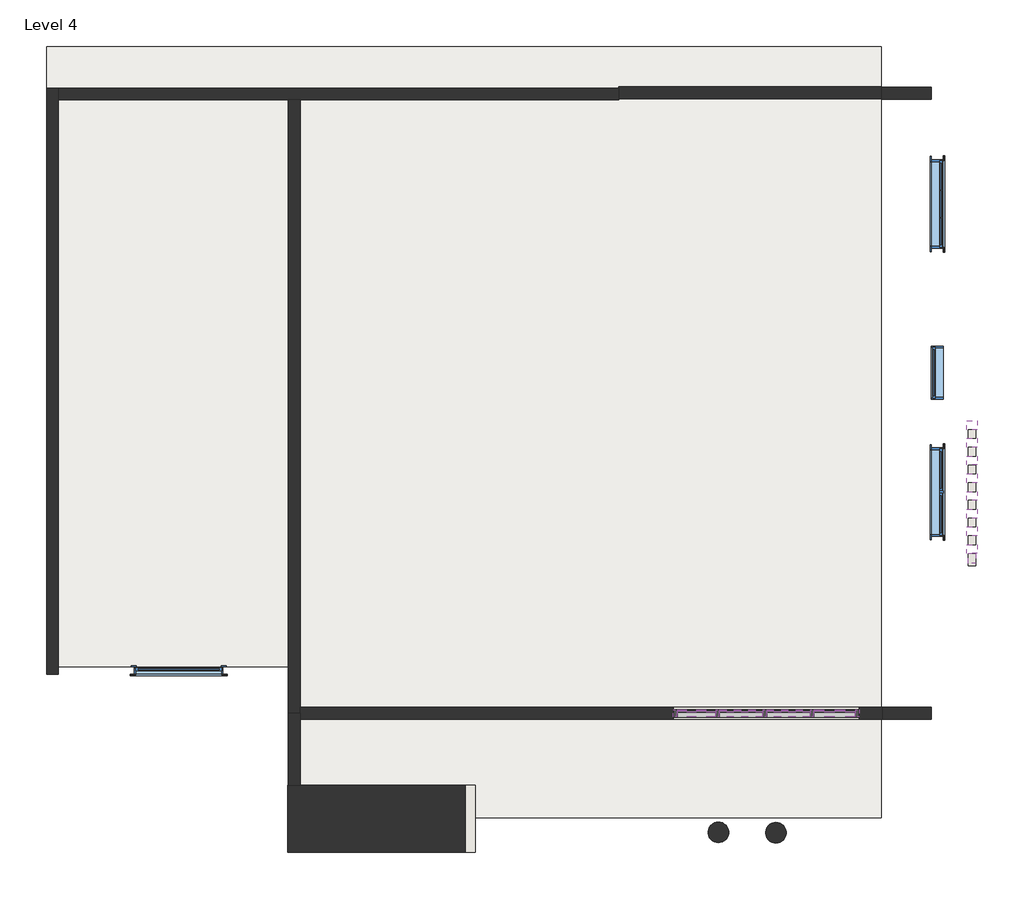
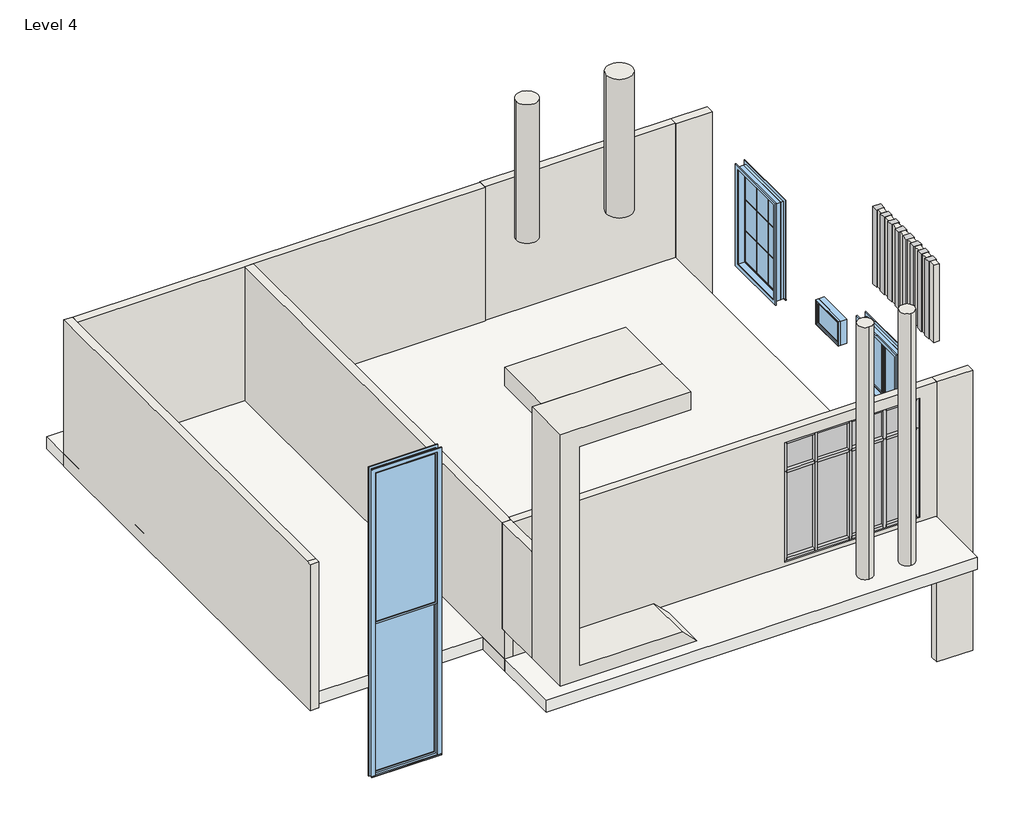
# One storey, incomplete: 22 members, 12 walls, 8 plates, 8 proxies, 4 windows, 1 roof.
"""IFC4 building model written with IfcOpenShell, lengths in millimetres."""

from ifc_helpers import new_model, si_unit, frame, origin, place, context, project, spatial, polyline, outline, extrude, faceted_brep, transform, mapped, element, save
from components import member_424e4c0f, member_61742b2b, member_5ade0aff, member_4d884067, member_c8ba4a72, member_20537117, member_aa870034, member_3a21dca5, member_2ee2964b, member_c33c434a, system_panel_glazed_10e47eeb, system_panel_glazed_d00a1739, system_panel_glazed_0ca22ccd, system_panel_glazed_ae16f783, system_panel_glazed_8c1b86c6, system_panel_glazed_afa25fb8, walls_4_walls_4_fad0a3e8, walls_5_walls_5_b947fde3, window_41dcc157, window_514a67b1, window_120b3672, window_57c3ee1c

model = new_model("IFC4")

# Units and contexts
model_context = context("Model", 3, world=origin())
ifc_project = project(units=[si_unit("LENGTHUNIT", "METRE", prefix="MILLI")], contexts=[model_context])

# Site, building, storey
site = spatial("IfcSite", under=ifc_project)
building = spatial("IfcBuilding", under=site)
storey = spatial("IfcBuildingStorey", under=building, Name="Level 4", Elevation=10972.8)

# Proxies
placement = place(None, origin())
element("IfcBuildingElementProxy", 1, Name="Reveal", ObjectType="Reveal", at=placement, inside=storey, context=model_context, shape_type="SweptSolid", body=[
    extrude(outline(polyline([(6653.2312442, 1993.3798743), (6470.3512442, 1993.3798743), (6470.3512442, 2145.7798743), (6653.2312442, 2145.7798743), (6653.2312442, 1993.3798743)])), frame((0.0, 0.0, 13469.4222175), z_axis=(0.0, 0.0, 1.0), x_axis=(1.0, 0.0, 0.0)), (0.0, 0.0, 1.0), 1931.5129026),
])
element("IfcBuildingElementProxy", 2, Name="Reveal", ObjectType="Reveal", at=placement, inside=storey, context=model_context, shape_type="SweptSolid", body=[
    extrude(outline(polyline([(6653.2312442, 2298.1798743), (6470.3512442, 2298.1798743), (6470.3512442, 2450.5798743), (6653.2312442, 2450.5798743), (6653.2312442, 2298.1798743)])), frame((0.0, 0.0, 13469.4222175), z_axis=(0.0, 0.0, 1.0), x_axis=(1.0, 0.0, 0.0)), (0.0, 0.0, 1.0), 1931.5129026),
])
element("IfcBuildingElementProxy", 3, Name="Reveal", ObjectType="Reveal", at=placement, inside=storey, context=model_context, shape_type="SweptSolid", body=[
    extrude(outline(polyline([(6653.2312442, 2602.9798743), (6470.3512442, 2602.9798743), (6470.3512442, 2755.3798743), (6653.2312442, 2755.3798743), (6653.2312442, 2602.9798743)])), frame((0.0, 0.0, 13469.4222175), z_axis=(0.0, 0.0, 1.0), x_axis=(1.0, 0.0, 0.0)), (0.0, 0.0, 1.0), 1931.5129026),
])
element("IfcBuildingElementProxy", 4, Name="Reveal", ObjectType="Reveal", at=placement, inside=storey, context=model_context, shape_type="SweptSolid", body=[
    extrude(outline(polyline([(6653.2312442, 2907.7798743), (6470.3512442, 2907.7798743), (6470.3512442, 3060.1798743), (6653.2312442, 3060.1798743), (6653.2312442, 2907.7798743)])), frame((0.0, 0.0, 13469.4222175), z_axis=(0.0, 0.0, 1.0), x_axis=(1.0, 0.0, 0.0)), (0.0, 0.0, 1.0), 1931.5129026),
])
element("IfcBuildingElementProxy", 5, Name="Reveal", ObjectType="Reveal", at=placement, inside=storey, context=model_context, shape_type="SweptSolid", body=[
    extrude(outline(polyline([(6653.2312442, 3212.5798743), (6470.3512442, 3212.5798743), (6470.3512442, 3364.9798743), (6653.2312442, 3364.9798743), (6653.2312442, 3212.5798743)])), frame((0.0, 0.0, 13469.4222175), z_axis=(0.0, 0.0, 1.0), x_axis=(1.0, 0.0, 0.0)), (0.0, 0.0, 1.0), 1931.5129026),
])
element("IfcBuildingElementProxy", 6, Name="Reveal", ObjectType="Reveal", at=placement, inside=storey, context=model_context, shape_type="SweptSolid", body=[
    extrude(outline(polyline([(6653.2312442, 3517.3798743), (6470.3512442, 3517.3798743), (6470.3512442, 3669.7798743), (6653.2312442, 3669.7798743), (6653.2312442, 3517.3798743)])), frame((0.0, 0.0, 13469.4222175), z_axis=(0.0, 0.0, 1.0), x_axis=(1.0, 0.0, 0.0)), (0.0, 0.0, 1.0), 1931.5129026),
])
element("IfcBuildingElementProxy", 7, Name="Reveal", ObjectType="Reveal", at=placement, inside=storey, context=model_context, shape_type="SweptSolid", body=[
    extrude(outline(polyline([(6653.2312442, 3822.1798743), (6470.3512442, 3822.1798743), (6470.3512442, 3974.5798743), (6653.2312442, 3974.5798743), (6653.2312442, 3822.1798743)])), frame((0.0, 0.0, 13469.4222175), z_axis=(0.0, 0.0, 1.0), x_axis=(1.0, 0.0, 0.0)), (0.0, 0.0, 1.0), 1931.5129026),
])
element("IfcBuildingElementProxy", 8, Name="Reveal", ObjectType="Reveal", at=placement, inside=storey, context=model_context, shape_type="SweptSolid", body=[
    extrude(outline(polyline([(6653.2312442, 4126.9798743), (6470.3512442, 4126.9798743), (6470.3512442, 4279.3798743), (6653.2312442, 4279.3798743), (6653.2312442, 4126.9798743)])), frame((0.0, 0.0, 13469.4222175), z_axis=(0.0, 0.0, 1.0), x_axis=(1.0, 0.0, 0.0)), (0.0, 0.0, 1.0), 1931.5129026),
])

# Members
member_shape = member_424e4c0f(model_context)
element("IfcMember", 9, ObjectType="Rectangular Mullion : 2.5\" x 5\" rectangular", at=placement, inside=storey, context=model_context, shape_type="MappedRepresentation", body=[
    mapped(member_shape, transform((3771.7551378, -759.3451257, 13606.9840877), x_axis=(0.0, 0.0, 1.0), y_axis=(0.0, -1.0, 0.0), z_axis=(1.0, 0.0, 0.0))),
])
element("IfcMember", 10, ObjectType="Rectangular Mullion : 2.5\" x 5\" rectangular", at=placement, inside=storey, context=model_context, shape_type="MappedRepresentation", body=[
    mapped(member_shape, transform((2958.9382617, -759.3451257, 13606.9840877), x_axis=(0.0, 0.0, 1.0), y_axis=(0.0, -1.0, 0.0), z_axis=(1.0, 0.0, 0.0))),
])
member_2_shape = member_61742b2b(model_context)
element("IfcMember", 11, ObjectType="Rectangular Mullion : 2.5\" x 5\" rectangular", at=placement, inside=storey, context=model_context, shape_type="MappedRepresentation", body=[
    mapped(member_2_shape, transform((2177.8713856, -759.3451257, 13606.9840877), x_axis=(1.0, 0.0, 0.0), y_axis=(0.0, -1.0, 0.0), z_axis=(0.0, 0.0, -1.0))),
])
element("IfcMember", 12, ObjectType="Rectangular Mullion : 2.5\" x 5\" rectangular", at=placement, inside=storey, context=model_context, shape_type="MappedRepresentation", body=[
    mapped(member_2_shape, transform((2990.6882617, -759.3451257, 13606.9840877), x_axis=(1.0, 0.0, 0.0), y_axis=(0.0, -1.0, 0.0), z_axis=(0.0, 0.0, -1.0))),
])
element("IfcMember", 13, ObjectType="Rectangular Mullion : 2.5\" x 5\" rectangular", at=placement, inside=storey, context=model_context, shape_type="MappedRepresentation", body=[
    mapped(member_2_shape, transform((3803.5051378, -759.3451257, 13606.9840877), x_axis=(1.0, 0.0, 0.0), y_axis=(0.0, -1.0, 0.0), z_axis=(0.0, 0.0, -1.0))),
])
member_3_shape = member_5ade0aff(model_context)
element("IfcMember", 14, ObjectType="Rectangular Mullion : 2.5\" x 5\" rectangular", at=placement, inside=storey, context=model_context, shape_type="MappedRepresentation", body=[
    mapped(member_3_shape, transform((3771.7551378, -759.3451257, 14368.9840877), x_axis=(0.0, 0.0, 1.0), y_axis=(0.0, -1.0, 0.0), z_axis=(1.0, 0.0, 0.0))),
])
element("IfcMember", 15, ObjectType="Rectangular Mullion : 2.5\" x 5\" rectangular", at=placement, inside=storey, context=model_context, shape_type="MappedRepresentation", body=[
    mapped(member_3_shape, transform((2958.9382617, -759.3451257, 14368.9840877), x_axis=(0.0, 0.0, 1.0), y_axis=(0.0, -1.0, 0.0), z_axis=(1.0, 0.0, 0.0))),
])
member_4_shape = member_4d884067(model_context)
element("IfcMember", 16, ObjectType="Rectangular Mullion : 2.5\" x 5\" rectangular", at=placement, inside=storey, context=model_context, shape_type="MappedRepresentation", body=[
    mapped(member_4_shape, transform((2177.8713856, -759.3451257, 11379.2), x_axis=(1.0, 0.0, 0.0), y_axis=(0.0, -1.0, 0.0), z_axis=(0.0, 0.0, -1.0))),
])
element("IfcMember", 17, ObjectType="Rectangular Mullion : 2.5\" x 5\" rectangular", at=placement, inside=storey, context=model_context, shape_type="MappedRepresentation", body=[
    mapped(member_4_shape, transform((2990.6882617, -759.3451257, 11379.2), x_axis=(1.0, 0.0, 0.0), y_axis=(0.0, -1.0, 0.0), z_axis=(0.0, 0.0, -1.0))),
])
element("IfcMember", 18, ObjectType="Rectangular Mullion : 2.5\" x 5\" rectangular", at=placement, inside=storey, context=model_context, shape_type="MappedRepresentation", body=[
    mapped(member_4_shape, transform((3803.5051378, -759.3451257, 11379.2), x_axis=(1.0, 0.0, 0.0), y_axis=(0.0, -1.0, 0.0), z_axis=(0.0, 0.0, -1.0))),
])
element("IfcMember", 19, ObjectType="Rectangular Mullion : 2.5\" x 5\" rectangular", at=placement, inside=storey, context=model_context, shape_type="MappedRepresentation", body=[
    mapped(member_3_shape, transform((3022.4382617, -759.3451257, 11379.2), x_axis=(0.0, 0.0, -1.0), y_axis=(0.0, -1.0, 0.0), z_axis=(-1.0, 0.0, 0.0))),
])
element("IfcMember", 20, ObjectType="Rectangular Mullion : 2.5\" x 5\" rectangular", at=placement, inside=storey, context=model_context, shape_type="MappedRepresentation", body=[
    mapped(member_3_shape, transform((2209.6213856, -759.3451257, 11379.2), x_axis=(0.0, 0.0, -1.0), y_axis=(0.0, -1.0, 0.0), z_axis=(-1.0, 0.0, 0.0))),
])
member_5_shape = member_c8ba4a72(model_context)
element("IfcMember", 21, ObjectType="Rectangular Mullion : 2.5\" x 5\" rectangular", at=placement, inside=storey, context=model_context, shape_type="MappedRepresentation", body=[
    mapped(member_5_shape, transform((4552.8220139, -759.3451257, 13606.9840877), x_axis=(0.0, 0.0, 1.0), y_axis=(0.0, -1.0, 0.0), z_axis=(1.0, 0.0, 0.0))),
])
member_6_shape = member_20537117(model_context)
element("IfcMember", 22, ObjectType="Rectangular Mullion : 2.5\" x 5\" rectangular", at=placement, inside=storey, context=model_context, shape_type="MappedRepresentation", body=[
    mapped(member_6_shape, transform((4552.8220139, -759.3451257, 14368.9840877), x_axis=(0.0, 0.0, 1.0), y_axis=(0.0, -1.0, 0.0), z_axis=(1.0, 0.0, 0.0))),
])
element("IfcMember", 23, ObjectType="Rectangular Mullion : 2.5\" x 5\" rectangular", at=placement, inside=storey, context=model_context, shape_type="MappedRepresentation", body=[
    mapped(member_6_shape, transform((3835.2551378, -759.3451257, 11379.2), x_axis=(0.0, 0.0, -1.0), y_axis=(0.0, -1.0, 0.0), z_axis=(-1.0, 0.0, 0.0))),
])
member_7_shape = member_aa870034(model_context)
element("IfcMember", 24, ObjectType="Rectangular Mullion : 2.5\" x 5\" rectangular", at=placement, inside=storey, context=model_context, shape_type="MappedRepresentation", body=[
    mapped(member_7_shape, transform((4616.3220139, -759.3451257, 13606.9840877), x_axis=(1.0, 0.0, 0.0), y_axis=(0.0, -1.0, 0.0), z_axis=(0.0, 0.0, -1.0))),
])
member_8_shape = member_3a21dca5(model_context)
element("IfcMember", 25, ObjectType="Rectangular Mullion : 2.5\" x 5\" rectangular", at=placement, inside=storey, context=model_context, shape_type="MappedRepresentation", body=[
    mapped(member_8_shape, transform((4616.3220139, -759.3451257, 11379.2), x_axis=(1.0, 0.0, 0.0), y_axis=(0.0, -1.0, 0.0), z_axis=(0.0, 0.0, -1.0))),
])
member_9_shape = member_2ee2964b(model_context)
element("IfcMember", 26, ObjectType="Rectangular Mullion : 2.5\" x 5\" rectangular", at=placement, inside=storey, context=model_context, shape_type="MappedRepresentation", body=[
    mapped(member_9_shape, transform((2146.1213856, -759.3451257, 13606.9840877), x_axis=(0.0, 0.0, 1.0), y_axis=(0.0, -1.0, 0.0), z_axis=(1.0, 0.0, 0.0))),
])
member_10_shape = member_c33c434a(model_context)
element("IfcMember", 27, ObjectType="Rectangular Mullion : 2.5\" x 5\" rectangular", at=placement, inside=storey, context=model_context, shape_type="MappedRepresentation", body=[
    mapped(member_10_shape, transform((2146.1213856, -759.3451257, 14368.9840877), x_axis=(0.0, 0.0, 1.0), y_axis=(0.0, -1.0, 0.0), z_axis=(1.0, 0.0, 0.0))),
])
element("IfcMember", 28, ObjectType="Rectangular Mullion : 2.5\" x 5\" rectangular", at=placement, inside=storey, context=model_context, shape_type="MappedRepresentation", body=[
    mapped(member_10_shape, transform((1479.3713856, -759.3451257, 11379.2), x_axis=(0.0, 0.0, -1.0), y_axis=(0.0, -1.0, 0.0), z_axis=(-1.0, 0.0, 0.0))),
])
element("IfcMember", 29, ObjectType="Rectangular Mullion : 2.5\" x 5\" rectangular", at=placement, inside=storey, context=model_context, shape_type="MappedRepresentation", body=[
    mapped(member_8_shape, transform((1415.8713856, -759.3451257, 13606.9840877), x_axis=(-1.0, 0.0, 0.0), y_axis=(0.0, -1.0, 0.0), z_axis=(0.0, 0.0, 1.0))),
])
element("IfcMember", 30, ObjectType="Rectangular Mullion : 2.5\" x 5\" rectangular", at=placement, inside=storey, context=model_context, shape_type="MappedRepresentation", body=[
    mapped(member_7_shape, transform((1415.8713856, -759.3451257, 14368.9840877), x_axis=(-1.0, 0.0, 0.0), y_axis=(0.0, -1.0, 0.0), z_axis=(0.0, 0.0, 1.0))),
])

# Plates
system_panel_glazed_shape = system_panel_glazed_10e47eeb(model_context)
element("IfcPlate", 31, ObjectType="System Panel : Glazed", at=placement, inside=storey, context=model_context, shape_type="MappedRepresentation", body=[
    mapped(system_panel_glazed_shape, transform((2584.2798237, -759.3451257, 13638.7340877), x_axis=(1.0, 0.0, 0.0), y_axis=(0.0, 1.0, 0.0), z_axis=(0.0, 0.0, 1.0))),
])
element("IfcPlate", 32, ObjectType="System Panel : Glazed", at=placement, inside=storey, context=model_context, shape_type="MappedRepresentation", body=[
    mapped(system_panel_glazed_shape, transform((3397.0966998, -759.3451257, 13638.7340877), x_axis=(1.0, 0.0, 0.0), y_axis=(0.0, 1.0, 0.0), z_axis=(0.0, 0.0, 1.0))),
])
system_panel_glazed_2_shape = system_panel_glazed_d00a1739(model_context)
element("IfcPlate", 33, ObjectType="System Panel : Glazed", at=placement, inside=storey, context=model_context, shape_type="MappedRepresentation", body=[
    mapped(system_panel_glazed_2_shape, transform((2584.2798237, -759.3451257, 11442.7), x_axis=(1.0, 0.0, 0.0), y_axis=(0.0, 1.0, 0.0), z_axis=(0.0, 0.0, 1.0))),
])
element("IfcPlate", 34, ObjectType="System Panel : Glazed", at=placement, inside=storey, context=model_context, shape_type="MappedRepresentation", body=[
    mapped(system_panel_glazed_2_shape, transform((3397.0966998, -759.3451257, 11442.7), x_axis=(1.0, 0.0, 0.0), y_axis=(0.0, 1.0, 0.0), z_axis=(0.0, 0.0, 1.0))),
])
system_panel_glazed_3_shape = system_panel_glazed_0ca22ccd(model_context)
element("IfcPlate", 35, ObjectType="System Panel : Glazed", at=placement, inside=storey, context=model_context, shape_type="MappedRepresentation", body=[
    mapped(system_panel_glazed_3_shape, transform((4194.0385758, -759.3451257, 11442.7), x_axis=(1.0, 0.0, 0.0), y_axis=(0.0, 1.0, 0.0), z_axis=(0.0, 0.0, 1.0))),
])
system_panel_glazed_4_shape = system_panel_glazed_ae16f783(model_context)
element("IfcPlate", 36, ObjectType="System Panel : Glazed", at=placement, inside=storey, context=model_context, shape_type="MappedRepresentation", body=[
    mapped(system_panel_glazed_4_shape, transform((4194.0385758, -759.3451257, 13638.7340877), x_axis=(1.0, 0.0, 0.0), y_axis=(0.0, 1.0, 0.0), z_axis=(0.0, 0.0, 1.0))),
])
system_panel_glazed_5_shape = system_panel_glazed_8c1b86c6(model_context)
element("IfcPlate", 37, ObjectType="System Panel : Glazed", at=placement, inside=storey, context=model_context, shape_type="MappedRepresentation", body=[
    mapped(system_panel_glazed_5_shape, transform((1812.7463856, -759.3451257, 11442.7), x_axis=(1.0, 0.0, 0.0), y_axis=(0.0, 1.0, 0.0), z_axis=(0.0, 0.0, 1.0))),
])
system_panel_glazed_6_shape = system_panel_glazed_afa25fb8(model_context)
element("IfcPlate", 38, ObjectType="System Panel : Glazed", at=placement, inside=storey, context=model_context, shape_type="MappedRepresentation", body=[
    mapped(system_panel_glazed_6_shape, transform((1812.7463856, -759.3451257, 13638.7340877), x_axis=(1.0, 0.0, 0.0), y_axis=(0.0, 1.0, 0.0), z_axis=(0.0, 0.0, 1.0))),
])

# Roof
element("IfcRoof", 39, ObjectType="Generic - 12\"", at=placement, inside=storey, context=model_context, shape_type="SweptSolid", body=[
    extrude(outline(polyline([(-9379.3749149, 10724.4481987), (4997.0250851, 10724.4481987), (4997.0250851, -2559.7518013), (-5213.7749149, -2559.7518013), (-5213.7749149, 40.7548743), (-9379.3749149, 40.7548743), (-9379.3749149, 10724.4481987)])), frame((0.0, 0.0, 10972.8), z_axis=(0.0, 0.0, 1.0), x_axis=(1.0, 0.0, 0.0)), (0.0, 0.0, 1.0), 304.8),
])

# Walls
element("IfcWall", 40, ObjectType="Generic - 5\"", at=placement, inside=storey, context=model_context, shape_type="SweptSolid", body=[
    extrude(outline(polyline([(6622.7512442, 1824.7794951), (6495.7512442, 1824.7794951), (6495.7512442, 1993.3798743), (6622.7512442, 1993.3798743), (6622.7512442, 1824.7794951)])), frame((0.0, 0.0, 13469.4222175), z_axis=(0.0, 0.0, 1.0), x_axis=(1.0, 0.0, 0.0)), (0.0, 0.0, 1.0), 1931.5129026),
    extrude(outline(polyline([(6622.7512442, 2145.7798743), (6495.7512442, 2145.7798743), (6495.7512442, 2298.1798743), (6622.7512442, 2298.1798743), (6622.7512442, 2145.7798743)])), frame((0.0, 0.0, 13469.4222175), z_axis=(0.0, 0.0, 1.0), x_axis=(1.0, 0.0, 0.0)), (0.0, 0.0, 1.0), 1931.5129026),
    extrude(outline(polyline([(6622.7512442, 2450.5798743), (6495.7512442, 2450.5798743), (6495.7512442, 2602.9798743), (6622.7512442, 2602.9798743), (6622.7512442, 2450.5798743)])), frame((0.0, 0.0, 13469.4222175), z_axis=(0.0, 0.0, 1.0), x_axis=(1.0, 0.0, 0.0)), (0.0, 0.0, 1.0), 1931.5129026),
    extrude(outline(polyline([(6622.7512442, 2755.3798743), (6495.7512442, 2755.3798743), (6495.7512442, 2907.7798743), (6622.7512442, 2907.7798743), (6622.7512442, 2755.3798743)])), frame((0.0, 0.0, 13469.4222175), z_axis=(0.0, 0.0, 1.0), x_axis=(1.0, 0.0, 0.0)), (0.0, 0.0, 1.0), 1931.5129026),
    extrude(outline(polyline([(6622.7512442, 3060.1798743), (6495.7512442, 3060.1798743), (6495.7512442, 3212.5798743), (6622.7512442, 3212.5798743), (6622.7512442, 3060.1798743)])), frame((0.0, 0.0, 13469.4222175), z_axis=(0.0, 0.0, 1.0), x_axis=(1.0, 0.0, 0.0)), (0.0, 0.0, 1.0), 1931.5129026),
    extrude(outline(polyline([(6622.7512442, 3364.9798743), (6495.7512442, 3364.9798743), (6495.7512442, 3517.3798743), (6622.7512442, 3517.3798743), (6622.7512442, 3364.9798743)])), frame((0.0, 0.0, 13469.4222175), z_axis=(0.0, 0.0, 1.0), x_axis=(1.0, 0.0, 0.0)), (0.0, 0.0, 1.0), 1931.5129026),
    extrude(outline(polyline([(6622.7512442, 3669.7798743), (6495.7512442, 3669.7798743), (6495.7512442, 3822.1798743), (6622.7512442, 3822.1798743), (6622.7512442, 3669.7798743)])), frame((0.0, 0.0, 13469.4222175), z_axis=(0.0, 0.0, 1.0), x_axis=(1.0, 0.0, 0.0)), (0.0, 0.0, 1.0), 1931.5129026),
    extrude(outline(polyline([(6622.7512442, 3974.5798743), (6495.7512442, 3974.5798743), (6495.7512442, 4126.9798743), (6622.7512442, 4126.9798743), (6622.7512442, 3974.5798743)])), frame((0.0, 0.0, 13469.4222175), z_axis=(0.0, 0.0, 1.0), x_axis=(1.0, 0.0, 0.0)), (0.0, 0.0, 1.0), 1931.5129026),
])
element("IfcWall", 41, ObjectType="Generic - 5\"", at=placement, inside=storey, context=model_context, shape_type="SweptSolid", body=[
    extrude(outline(polyline([(6622.7512442, 1784.3255336), (6495.7512442, 1784.3255336), (6495.7512442, 1993.3798743), (6622.7512442, 1993.3798743), (6622.7512442, 1784.3255336)])), frame((0.0, 0.0, 7620.0), z_axis=(0.0, 0.0, 1.0), x_axis=(1.0, 0.0, 0.0)), (0.0, 0.0, 1.0), 2067.2126797),
    extrude(outline(polyline([(6622.7512442, 2145.7798743), (6495.7512442, 2145.7798743), (6495.7512442, 2298.1798743), (6622.7512442, 2298.1798743), (6622.7512442, 2145.7798743)])), frame((0.0, 0.0, 7620.0), z_axis=(0.0, 0.0, 1.0), x_axis=(1.0, 0.0, 0.0)), (0.0, 0.0, 1.0), 2067.2126797),
    extrude(outline(polyline([(6622.7512442, 2450.5798743), (6495.7512442, 2450.5798743), (6495.7512442, 2602.9798743), (6622.7512442, 2602.9798743), (6622.7512442, 2450.5798743)])), frame((0.0, 0.0, 7620.0), z_axis=(0.0, 0.0, 1.0), x_axis=(1.0, 0.0, 0.0)), (0.0, 0.0, 1.0), 2067.2126797),
    extrude(outline(polyline([(6622.7512442, 2755.3798743), (6495.7512442, 2755.3798743), (6495.7512442, 2907.7798743), (6622.7512442, 2907.7798743), (6622.7512442, 2755.3798743)])), frame((0.0, 0.0, 7620.0), z_axis=(0.0, 0.0, 1.0), x_axis=(1.0, 0.0, 0.0)), (0.0, 0.0, 1.0), 2067.2126797),
    extrude(outline(polyline([(6622.7512442, 3060.1798743), (6495.7512442, 3060.1798743), (6495.7512442, 3212.5798743), (6622.7512442, 3212.5798743), (6622.7512442, 3060.1798743)])), frame((0.0, 0.0, 7620.0), z_axis=(0.0, 0.0, 1.0), x_axis=(1.0, 0.0, 0.0)), (0.0, 0.0, 1.0), 2067.2126797),
    extrude(outline(polyline([(6622.7512442, 3364.9798743), (6495.7512442, 3364.9798743), (6495.7512442, 3517.3798743), (6622.7512442, 3517.3798743), (6622.7512442, 3364.9798743)])), frame((0.0, 0.0, 7620.0), z_axis=(0.0, 0.0, 1.0), x_axis=(1.0, 0.0, 0.0)), (0.0, 0.0, 1.0), 2067.2126797),
    extrude(outline(polyline([(6622.7512442, 3669.7798743), (6495.7512442, 3669.7798743), (6495.7512442, 3822.1798743), (6622.7512442, 3822.1798743), (6622.7512442, 3669.7798743)])), frame((0.0, 0.0, 7620.0), z_axis=(0.0, 0.0, 1.0), x_axis=(1.0, 0.0, 0.0)), (0.0, 0.0, 1.0), 2067.2126797),
    extrude(outline(polyline([(6622.7512442, 3974.5798743), (6495.7512442, 3974.5798743), (6495.7512442, 4126.9798743), (6622.7512442, 4126.9798743), (6622.7512442, 3974.5798743)])), frame((0.0, 0.0, 7620.0), z_axis=(0.0, 0.0, 1.0), x_axis=(1.0, 0.0, 0.0)), (0.0, 0.0, 1.0), 2067.2126797),
])
element("IfcWall", 42, ObjectType="Generic - 8\"", at=placement, inside=storey, context=model_context, shape_type="Brep", body=[
    faceted_brep([(5860.6250851, -657.7451257, 7620.0), (5016.0750851, -657.7451257, 7620.0), (5016.0750851, -657.7451257, 10972.8), (5016.0750851, -657.7451257, 14630.4), (5860.6250851, -657.7451257, 14630.4), (5860.6250851, -860.9451257, 7620.0), (5860.6250851, -860.9451257, 14630.4), (5016.0750851, -860.9451257, 14630.4), (5016.0750851, -860.9451257, 10972.8), (5016.0750851, -860.9451257, 7620.0)], [[[0, 1, 2, 3, 4]], [[5, 6, 7, 8, 9]], [[1, 0, 5, 9]], [[0, 4, 6, 5]], [[4, 3, 7, 6]], [[1, 9, 8, 7, 3, 2]]]),
])
element("IfcWall", 43, ObjectType="Generic - 8\"", at=placement, inside=storey, context=model_context, shape_type="SweptSolid", body=[
    extrude(outline(polyline([(4997.0250851, 10019.7798743), (5860.6250851, 10019.7798743), (5860.6250851, 9816.5798743), (4997.0250851, 9816.5798743), (4997.0250851, 10019.7798743)])), frame((0.0, 0.0, 7620.0), z_axis=(0.0, 0.0, 1.0), x_axis=(1.0, 0.0, 0.0)), (0.0, 0.0, 1.0), 7010.4),
])
element("IfcWall", 44, ObjectType="Generic - 8\"", at=placement, inside=storey, context=model_context, shape_type="Brep", body=[
    faceted_brep([(-5010.5749149, -860.9451257, 10972.8), (-5010.5749149, -657.7451257, 10972.8), (-5010.5749149, 9807.0548743, 10972.8), (-5010.5749149, 9807.0548743, 14630.4), (-5010.5749149, -657.7451257, 14630.4), (-5010.5749149, -759.3451257, 14630.4), (-5010.5749149, -759.3451257, 11976.102518), (-5010.5749149, -860.9451257, 11976.102518), (-5213.7749149, -860.9451257, 10972.8), (-5213.7749149, -860.9451257, 11976.102518), (-5213.7749149, -759.3451257, 11976.102518), (-5213.7749149, -759.3451257, 14630.4), (-5213.7749149, 40.7548743, 14630.4), (-5213.7749149, 9807.0548743, 14630.4), (-5213.7749149, 9807.0548743, 10972.8)], [[[0, 1, 2, 3, 4, 5, 6, 7]], [[8, 9, 10, 11, 12, 13, 14]], [[2, 1, 0, 8, 14]], [[5, 4, 3, 13, 12, 11]], [[6, 5, 11, 10]], [[6, 10, 9, 7]], [[0, 7, 9, 8]], [[3, 2, 14, 13]]]),
])
element("IfcWall", 45, ObjectType="Generic - 8\"", at=placement, inside=storey, context=model_context, shape_type="Brep", body=[
    faceted_brep([(-9176.1749149, -86.2451257, 10972.8), (-9176.1749149, 9807.0548743, 10972.8), (-9176.1749149, 10010.2548743, 10972.8), (-9176.1749149, 10010.2548743, 14630.4), (-9176.1749149, 9807.0548743, 14630.4), (-9176.1749149, 40.7548743, 14630.4), (-9176.1749149, -86.2451257, 14630.4), (-9379.3749149, -86.2451257, 10972.8), (-9379.3749149, -86.2451257, 14630.4), (-9379.3749149, 40.7548743, 14630.4), (-9379.3749149, 10010.2548743, 14630.4), (-9379.3749149, 10010.2548743, 10972.8)], [[[0, 1, 2, 3, 4, 5, 6]], [[7, 8, 9, 10, 11]], [[2, 1, 0, 7, 11]], [[0, 6, 8, 7]], [[6, 5, 9, 8]], [[5, 4, 3, 10, 9]], [[3, 2, 11, 10]]]),
])
element("IfcWall", 46, ObjectType="Generic - 8\"", at=placement, inside=storey, context=model_context, shape_type="Brep", body=[
    faceted_brep([(-5213.7749149, -759.3451257, 11976.102518), (-5213.7749149, -860.9451257, 11976.102518), (-5213.7749149, -2002.282557, 11976.102518), (-5213.7749149, -2002.282557, 14630.4), (-5213.7749149, -759.3451257, 14630.4), (-5010.5749149, -759.3451257, 11976.102518), (-5010.5749149, -759.3451257, 14630.4), (-5010.5749149, -860.9451257, 14630.4), (-5010.5749149, -2002.282557, 14630.4), (-5010.5749149, -2002.282557, 11976.102518), (-5010.5749149, -860.9451257, 11976.102518)], [[[0, 1, 2, 3, 4]], [[5, 6, 7, 8, 9, 10]], [[2, 1, 0, 5, 10, 9]], [[3, 2, 9, 8]], [[4, 3, 8, 7, 6]], [[0, 4, 6, 5]]]),
])
element("IfcWall", 47, ObjectType="Generic - 8\"", at=placement, inside=storey, context=model_context, shape_type="Brep", body=[
    faceted_brep([(-5010.5749149, -657.7451257, 10972.8), (-5010.5749149, -657.7451257, 14630.4), (5016.0750851, -657.7451257, 14630.4), (5016.0750851, -657.7451257, 10972.8), (4616.3220139, -657.7451257, 14368.9840877), (1415.8713856, -657.7451257, 14368.9840877), (1415.8713856, -657.7451257, 11379.2), (4616.3220139, -657.7451257, 11379.2), (-5010.5749149, -860.9451257, 14630.4), (-5010.5749149, -860.9451257, 11976.102518), (-5010.5749149, -860.9451257, 10972.8), (5016.0750851, -860.9451257, 10972.8), (5016.0750851, -860.9451257, 14630.4), (4616.3220139, -860.9451257, 14368.9840877), (4616.3220139, -860.9451257, 11379.2), (1415.8713856, -860.9451257, 11379.2), (1415.8713856, -860.9451257, 14368.9840877), (-5010.5749149, -759.3451257, 14630.4)], [[[0, 1, 2, 3], [4, 5, 6, 7]], [[8, 9, 10, 11, 12], [13, 14, 15, 16]], [[0, 3, 11, 10]], [[3, 2, 12, 11]], [[2, 1, 17, 8, 12]], [[5, 4, 13, 16]], [[6, 5, 16, 15]], [[7, 6, 15, 14]], [[4, 7, 14, 13]], [[0, 10, 9, 8, 17, 1]]]),
])
element("IfcWall", 48, ObjectType="Generic - 8\"", at=placement, inside=storey, context=model_context, shape_type="Brep", body=[
    faceted_brep([(-9176.1749149, 9807.0548743, 10972.8), (-5213.7749149, 9807.0548743, 10972.8), (-5010.5749149, 9807.0548743, 10972.8), (475.8250851, 9807.0548743, 10972.8), (475.8250851, 9807.0548743, 14630.4), (-5010.5749149, 9807.0548743, 14630.4), (-5213.7749149, 9807.0548743, 14630.4), (-9176.1749149, 9807.0548743, 14630.4), (-9176.1749149, 10010.2548743, 10972.8), (-9176.1749149, 10010.2548743, 14630.4), (475.8250851, 10010.2548743, 14630.4), (475.8250851, 10010.2548743, 10972.8), (475.8250851, 9826.1048743, 10972.8), (475.8250851, 9826.1048743, 14630.4)], [[[0, 1, 2, 3, 4, 5, 6, 7]], [[8, 9, 10, 11]], [[3, 2, 1, 0, 8, 11, 12]], [[4, 3, 12, 11, 10, 13]], [[7, 6, 5, 4, 13, 10, 9]], [[0, 7, 9, 8]]]),
])
element("IfcWall", 49, ObjectType="Generic - 8\"", at=placement, inside=storey, context=model_context, shape_type="Brep", body=[
    faceted_brep([(475.8250851, 9826.1048743, 10972.8), (577.4250851, 9826.1048743, 10972.8), (4997.0250851, 9826.1048743, 10972.8), (4997.0250851, 9826.1048743, 14630.4), (475.8250851, 9826.1048743, 14630.4), (475.8250851, 10029.3048743, 10972.8), (475.8250851, 10029.3048743, 14630.4), (4997.0250851, 10029.3048743, 14630.4), (4997.0250851, 10029.3048743, 10972.8), (577.4250851, 10029.3048743, 10972.8), (475.8250851, 10010.2548743, 10972.8), (475.8250851, 10010.2548743, 14630.4)], [[[0, 1, 2, 3, 4]], [[5, 6, 7, 8, 9]], [[2, 1, 0, 10, 5, 9, 8]], [[0, 4, 11, 6, 5, 10]], [[3, 2, 8, 7]], [[4, 3, 7, 6, 11]]]),
])
walls_4_walls_4_shape = walls_4_walls_4_fad0a3e8(model_context)
element("IfcWall", 50, ObjectType="Walls 4 : Walls 4", at=placement, inside=storey, context=model_context, shape_type="MappedRepresentation", body=[
    mapped(walls_4_walls_4_shape, transform((0.0, 0.0, 0.0), x_axis=(1.0, 0.0, 0.0), y_axis=(0.0, 1.0, 0.0), z_axis=(0.0, 0.0, 1.0))),
])
walls_5_walls_5_shape = walls_5_walls_5_b947fde3(model_context)
element("IfcWall", 51, ObjectType="Walls 5 : Walls 5", at=placement, inside=storey, context=model_context, shape_type="MappedRepresentation", body=[
    mapped(walls_5_walls_5_shape, transform((0.0, 0.0, 0.0), x_axis=(1.0, 0.0, 0.0), y_axis=(0.0, 1.0, 0.0), z_axis=(0.0, 0.0, 1.0))),
])

# Windows
window_shape = window_41dcc157(model_context)
element("IfcWindow", 52, ObjectType="Casement 3x3 with Trim : 60\" x 96\"", at=placement, inside=storey, context=model_context, shape_type="MappedRepresentation", body=[
    mapped(window_shape, transform((5962.2250851, 8013.1798743, 11125.2), x_axis=(0.0, -1.0, 0.0), y_axis=(1.0, 0.0, 0.0), z_axis=(0.0, 0.0, 1.0))),
])
window_2_shape = window_514a67b1(model_context)
element("IfcWindow", 53, ObjectType="Casement Dbl with Trim : 60\" x 60\"", at=placement, inside=storey, context=model_context, shape_type="MappedRepresentation", body=[
    mapped(window_2_shape, transform((5943.1750851, 3050.6548743, 10639.8899453), x_axis=(0.0, -1.0, 0.0), y_axis=(1.0, 0.0, 0.0), z_axis=(0.0, 0.0, 1.0))),
])
window_3_shape = window_120b3672(model_context)
element("IfcWindow", 54, ObjectType="Double Hung with Trim : 60\" x 300\"", at=placement, inside=storey, context=model_context, shape_type="MappedRepresentation", body=[
    mapped(window_3_shape, transform((-7102.8999149, -22.7451257, 7885.5445366), x_axis=(-1.0, 0.0, 0.0), y_axis=(0.0, -1.0, 0.0), z_axis=(0.0, 0.0, 1.0))),
])
window_4_shape = window_57c3ee1c(model_context)
element("IfcWindow", 55, ObjectType="Fixed : 36\" x 24\"", at=placement, inside=storey, context=model_context, shape_type="MappedRepresentation", body=[
    mapped(window_4_shape, transform((5962.2250851, 5146.1548743, 10972.8), x_axis=(0.0, 1.0, 0.0), y_axis=(-1.0, 0.0, 0.0), z_axis=(0.0, 0.0, 1.0))),
])

save(model, "model.ifc")

# Revit data of these elements
# Type "Rectangular Mullion : 2.5\" x 5\" rectangular"
#   built-in parameter 1007304 = 0.416667 (stored number, unit not read)
#   built-in parameter 1007301 = 0.104167 (stored number, unit not read)
#   built-in parameter 1007300 = 0.104167 (stored number, unit not read)
# Type "System Panel : Glazed"
#   Construction Type Id = "GSP4R"
#   Analytic Construction = "1/8 in Pilkington single glazing"
#   Visual Light Transmittance = 0.9
#   Solar Heat Gain Coefficient = 0.86
#   Heat Transfer Coefficient (U) = 1.18115 BTU/(h·ft²·°F)
# Type "Generic - 12\""
#   Assembly Code = "B1020"
#   Layers, outside or top first: 1' - 0" no material (function 1)
# Type "Generic - 5\""
#   Assembly Code = "B2010"
#   Layers, outside or top first: 0' - 5" no material (function 1)
# Type "Generic - 8\""
#   Assembly Code = "B2010"
#   Layers, outside or top first: 0' - 8" no material (function 1)
# Type "Casement 3x3 with Trim : 60\" x 96\""
#   Type Mark = "15"
#   Construction Type Id = "GSP4R"
#   Assembly Code = "B2020100"
#   Analytic Construction = "1/8 in Pilkington single glazing"
#   Visual Light Transmittance = 0.9
#   Solar Heat Gain Coefficient = 0.78
#   Heat Transfer Coefficient (U) = 0.6496 BTU/(h·ft²·°F)
#   Height = 8' - 0"
#   Default Sill Height = 1' - 0"
#   Trim Projection - Ext. = 0' - 0 1/2"
#   Trim Projection - Int. = 0' - 0 3/4"
#   Trim Width - Exterior = 0' - 3 1/2"
#   Trim Width - Interior = 0' - 3 1/2"
#   Width = 5' - 0"
#   Window Inset = 0' - 0 3/4"
#   Define Thermal Properties by = 1
#   Glass Pane Material = Glass
#   Sash Material = Sash
#   Trim Exterior Material = Trim
#   Trim Interior Material = Trim
#   Wall Closure = (empty or 0)
# Type "Casement Dbl with Trim : 60\" x 60\""
#   Type Mark = "10"
#   Construction Type Id = "GSP4R"
#   Assembly Code = "B2020100"
#   Analytic Construction = "1/8 in Pilkington single glazing"
#   Visual Light Transmittance = 0.9
#   Thermal Resistance (R) = 1.53941 (h·ft²·°F)/BTU
#   Solar Heat Gain Coefficient = 0.78
#   Heat Transfer Coefficient (U) = 0.6496 BTU/(h·ft²·°F)
#   Height = 5' - 0"
#   Default Sill Height = 3' - 0"
#   Trim Projection - Ext. = 0' - 0 1/2"
#   Trim Projection - Int. = 0' - 0 3/4"
#   Trim Width - Exterior = 0' - 3 1/2"
#   Trim Width - Interior = 0' - 3 1/2"
#   Width = 5' - 0"
#   Window Inset = 0' - 0 3/4"
#   Define Thermal Properties by = 1
#   Glass Pane Material = Glass
#   Sash Material = Sash
#   Trim Exterior Material = Trim
#   Trim Interior Material = Roofing, EPDM Membrane
#   Wall Closure = (empty or 0)
# Type "Double Hung with Trim : 60\" x 300\""
#   Type Mark = "28"
#   Construction Type Id = "GSP4R"
#   Assembly Code = "B2020100"
#   Analytic Construction = "1/8 in Pilkington single glazing"
#   Visual Light Transmittance = 0.9
#   Solar Heat Gain Coefficient = 0.78
#   Heat Transfer Coefficient (U) = 0.6496 BTU/(h·ft²·°F)
#   Height = 25' - 0"
#   Default Sill Height = 3' - 0"
#   Trim Projection - Ext. = 0' - 0 1/2"
#   Trim Projection - Int. = 0' - 0 3/4"
#   Trim Width - Exterior = 0' - 3 1/2"
#   Trim Width - Interior = 0' - 3 1/2"
#   Width = 5' - 0"
#   Window Inset = 0' - 0 3/4"
#   Define Thermal Properties by = 1
#   Glass Pane Material = Glass
#   Sash Material = Sash
#   Trim Exterior Material = Trim
#   Trim Interior Material = Trim
#   Wall Closure = (empty or 0)
# Type "Fixed : 36\" x 24\""
#   Type Mark = "8"
#   Construction Type Id = "GSP4R"
#   Assembly Code = "B2020100"
#   Analytic Construction = "1/8 in Pilkington single glazing"
#   Visual Light Transmittance = 0.9
#   Solar Heat Gain Coefficient = 0.78
#   Heat Transfer Coefficient (U) = 0.6496 BTU/(h·ft²·°F)
#   Height = 2' - 0"
#   Default Sill Height = 3' - 0"
#   Width = 3' - 0"
#   Window Inset = 0' - 0 3/4"
#   Define Thermal Properties by = 1
#   Glass Pane Material = Glass
#   Sash Material = Sash
#   Wall Closure = (empty or 0)
# Elements 9, 10, 11, 12, 13, 14, 15, 16, 17, 18, 19, 20, 21, 22, 23, 24, 25, 26, 27, 28, 29, 30 (IfcMember, "Rectangular Mullion : 2.5\" x 5\" rectangular")
#   Phase Created = New Construction
#   Materials on its faces: "Aluminum"
# Elements 31, 32, 33, 34, 35, 36, 37, 38 (IfcPlate, "System Panel : Glazed")
#   Phase Created = New Construction
#   Materials on its faces: "Glass"
# Element 39 (IfcRoof, "Generic - 12\"")
#   built-in parameter 1001705 = 37 (stored number, unit not read)
#   built-in parameter 1001710 = 33615
#   Phase Created = New Construction
#   Materials on its faces: "Default Roof"
# Element 40 (IfcWall, "Generic - 5\"")
#   built-in parameter 1001111 = 8' - 2.29221"
#   Top Offset = 2' - 6.33603"
#   Base Offset = 8' - 2.29221"
#   wall height = 6' - 4.04382"
#   Phase Created = New Construction
#   Base Constraint = Level 4
#   Top Constraint = Level 5
#   Materials on its faces: "Default Wall"
# Element 41 (IfcWall, "Generic - 5\"")
#   built-in parameter 1001111 = -11' - 0"
#   Top Offset = -16' - 2.61367"
#   Base Offset = -11' - 0"
#   wall height = 6' - 9.38633"
#   Phase Created = New Construction
#   Base Constraint = Level 4
#   Top Constraint = Level 5
#   Materials on its faces: "Default Wall"
# Element 42 (IfcWall, "Generic - 8\"")
#   built-in parameter 1001111 = -11' - 0"
#   Top Offset = 0' - 0"
#   Base Offset = -11' - 0"
#   Unconnected Height = 23' - 1.65293"
#   wall height = 23' - 1.65293"
#   Phase Created = New Construction
#   Base Constraint = Level 4
#   Materials on its faces: "Default Wall"
# Element 43 (IfcWall, "Generic - 8\"")
#   built-in parameter 1001111 = -11' - 0"
#   Top Offset = 0' - 0"
#   Base Offset = -11' - 0"
#   Unconnected Height = 23' - 0"
#   wall height = 23' - 0"
#   Phase Created = New Construction
#   Base Constraint = Level 4
#   Materials on its faces: "Default Wall"
# Elements 44, 45, 47, 48, 49 (IfcWall, "Generic - 8\"")
#   Top Offset = 0' - 0"
#   Base Offset = 0' - 0"
#   Unconnected Height = 12' - 0"
#   wall height = 12' - 0"
#   Phase Created = New Construction
#   Base Constraint = Level 4
#   Materials on its faces: "Default Wall"
# Element 46 (IfcWall, "Generic - 8\"")
#   built-in parameter 1001111 = 3' - 3.5001"
#   Top Offset = 0' - 0"
#   Base Offset = 3' - 3.5001"
#   Unconnected Height = 8' - 8.4999"
#   wall height = 8' - 8.4999"
#   Phase Created = New Construction
#   Base Constraint = Level 4
#   Materials on its faces: "Default Wall"
# Element 50 (IfcWall, "Walls 4 : Walls 4")
#   Phase Created = New Construction
#   Materials on its faces: "Default Wall"
# Element 51 (IfcWall, "Walls 5 : Walls 5")
#   Phase Created = New Construction
#   Materials on its faces: "Default Wall"
# Element 52 (IfcWindow, "Casement 3x3 with Trim : 60\" x 96\"")
#   Mark = "2"
#   Phase Created = New Construction
#   Materials on its faces: "Sash", "Glass", "Trim"
# Element 53 (IfcWindow, "Casement Dbl with Trim : 60\" x 60\"")
#   Mark = "1"
#   Phase Created = New Construction
#   Materials on its faces: "Sash", "Trim", "Glass", "Roofing, EPDM Membrane"
# Element 54 (IfcWindow, "Double Hung with Trim : 60\" x 300\"")
#   Mark = "10"
#   Phase Created = New Construction
#   Materials on its faces: "Sash", "Trim", "Glass"
# Element 55 (IfcWindow, "Fixed : 36\" x 24\"")
#   Mark = "4"
#   Phase Created = New Construction
#   Materials on its faces: "Sash", "Glass"
# Materials
#   "Glass": class "Glass", colour RGB 0 128 192, transparency 0.75, Description = "Soda Lime Glass", Cost = 0
#   "Sash": class "Wood", colour RGB 224 178 126, transparency 0
#   "Trim": class "Wood", colour RGB 224 178 126, transparency 0
#   "Roofing, EPDM Membrane": class "Generic", colour RGB 127 127 127, transparency 0, Description = "EPDM roof membrane", Cost = 0
#   "Aluminum": class "Metal", colour RGB 247 247 247, transparency 0, Description = "Aluminum 6061", Cost = 0
#   "Default Roof": colour RGB 88 101 114, transparency 0
#   "Default Wall": colour RGB 128 128 128, transparency 0
